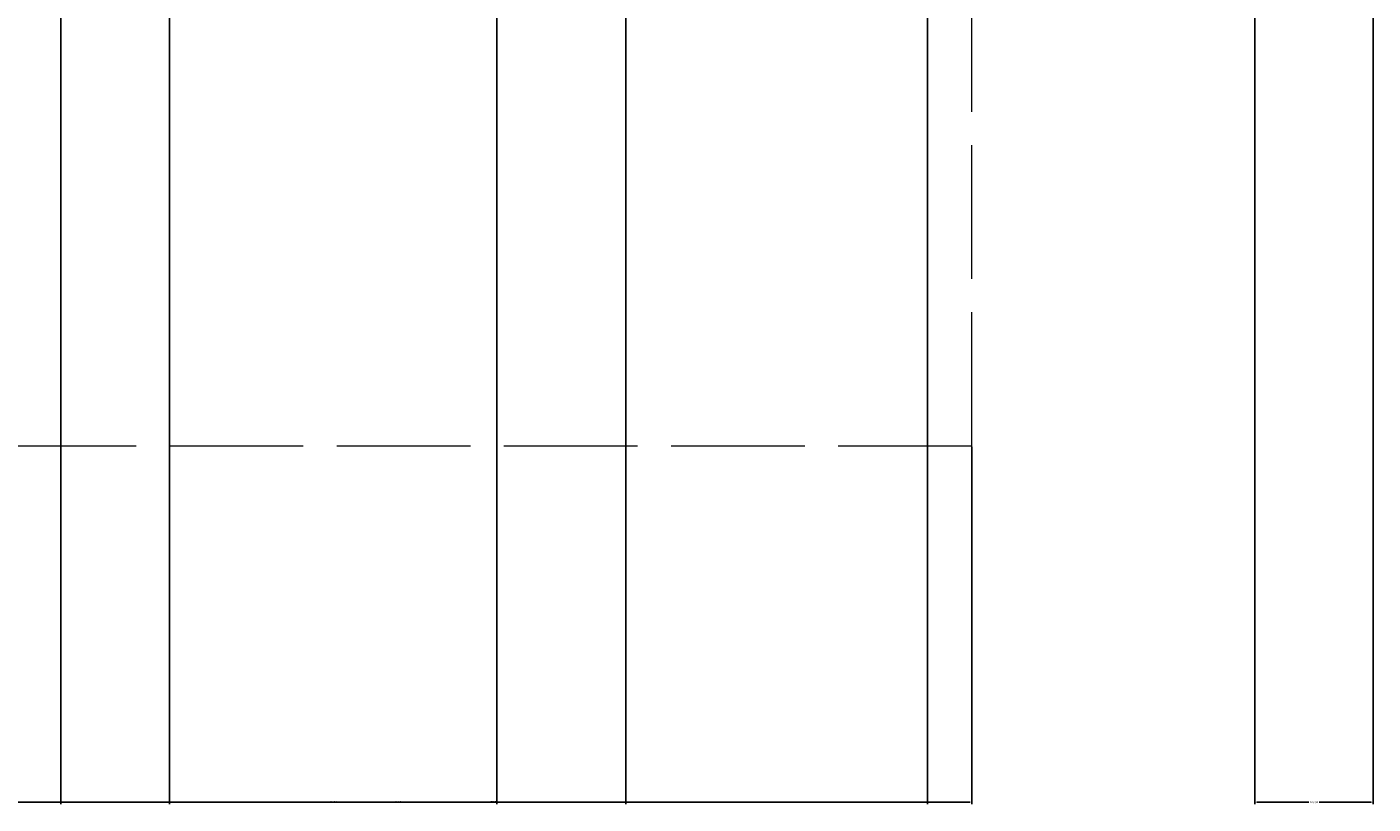
# Model space of a CAD drawing. Units: feet. Extents: x 1993 to 2298, y 2938 to 3641.
# Tile 2 of 11: x 2137 to 2258, y 2938 to 3008. Entities that reach past the tile are written whole.
import ezdxf

# ---------------------------------------------------------------- set-up
doc = ezdxf.new("R2010")
doc.units = ezdxf.units.FT
doc.linetypes.add('ACAD_ISO02W100', pattern=[15, 12, -3])
doc.layers.add('A-ANNO-DIMS', color=2, linetype='Continuous', lineweight=18)
doc.layers.add('SUNSHADES', color=4, linetype='ACAD_ISO02W100', lineweight=13)
doc.styles.get("Standard").update_dxf_attribs({"font": 'arial.ttf'})
doc.dimstyles.get("Standard").update_dxf_attribs({"dimtxt": 0.18, "dimasz": 0.18, "dimexe": 0.18, "dimexo": 0.0625, "dimgap": 0.09, "dimtad": 0, "dimtih": 1, "dimtoh": 1, "dimdec": 4, "dimzin": 0, "dimdsep": 46, "dimtxsty": 'Standard', "dimcen": 0.09, "dimadec": 0, "dimazin": 0, "dimtfac": 1, "dimtdec": 4, "dimtofl": 0, "dimtmove": 0, "dimatfit": 3, "dimfxl": 1, "dimtolj": 1, "dimtzin": 0, "dimarcsym": 0})

# ---------------------------------------------------------------- blocks, each defined once
blk = doc.blocks.new('*D57')
at = {"layer": 'A-ANNO-DIMS', "color": 0, "lineweight": -2, "transparency": 16777216}
for p, q in [((2029.76, 2969.94), (2029.76, 2937.86)), ((2221.76, 2969.94), (2221.76, 2937.86)), ((2029.94, 2938.03), (2125.48, 2938.03)), ((2221.58, 2938.03), (2126.04, 2938.03))]:
    blk.add_line(p, q, dxfattribs=at)
at = {"layer": 'A-ANNO-DIMS', "color": 0, "transparency": 16777216}
for points in [[(2029.94, 2938.07), (2029.94, 2938.01), (2029.76, 2938.03)], [(2221.58, 2938.07), (2221.58, 2938.01), (2221.76, 2938.03)]]:
    blk.add_solid(points, dxfattribs=at)
at = {"layer": 'Defpoints', "color": 0, "transparency": 16777216}
for p in [(2029.76, 2970), (2221.76, 2970), (2221.76, 2938.03)]:
    blk.add_point(p, dxfattribs=at)
at = {"layer": 'A-ANNO-DIMS', "color": 0, "transparency": 16777216, "insert": (2125.76, 2938.03), "char_height": 0.18, "attachment_point": 5}
blk.add_mtext('\\A1;192', dxfattribs=at)
blk = doc.blocks.new('*D60')
at = {"layer": 'A-ANNO-DIMS', "color": 0, "lineweight": -2, "transparency": 16777216}
for p, q in [((2140, 3012.47), (2140, 2937.86)), ((2217.76, 3012.47), (2217.76, 2937.86)), ((2140.18, 2938.03), (2178.49, 2938.03)), ((2217.58, 2938.03), (2179.27, 2938.03))]:
    blk.add_line(p, q, dxfattribs=at)
at = {"layer": 'A-ANNO-DIMS', "color": 0, "transparency": 16777216}
for points in [[(2140.18, 2938.07), (2140.18, 2938.01), (2140, 2938.03)], [(2217.58, 2938.07), (2217.58, 2938.01), (2217.76, 2938.03)]]:
    blk.add_solid(points, dxfattribs=at)
at = {"layer": 'Defpoints', "color": 0, "transparency": 16777216}
for p in [(2140, 3012.53), (2217.76, 3012.53), (2217.76, 2938.03)]:
    blk.add_point(p, dxfattribs=at)
at = {"layer": 'A-ANNO-DIMS', "color": 0, "transparency": 16777216, "insert": (2178.88, 2938.03), "char_height": 0.18, "attachment_point": 5}
blk.add_mtext('\\A1;77.76', dxfattribs=at)
blk = doc.blocks.new('*D65')
at = {"layer": 'A-ANNO-DIMS', "color": 0, "lineweight": -2, "transparency": 16777216}
for p, q in [((2179.12, 3231.85), (2179.12, 2937.86)), ((2149.76, 3228.47), (2149.76, 2937.86)), ((2149.94, 2938.03), (2164.04, 2938.03)), ((2178.94, 2938.03), (2164.83, 2938.03))]:
    blk.add_line(p, q, dxfattribs=at)
at = {"layer": 'A-ANNO-DIMS', "color": 0, "transparency": 16777216}
for points in [[(2149.94, 2938.07), (2149.94, 2938.01), (2149.76, 2938.03)], [(2178.94, 2938.07), (2178.94, 2938.01), (2179.12, 2938.03)]]:
    blk.add_solid(points, dxfattribs=at)
at = {"layer": 'Defpoints', "color": 0, "transparency": 16777216}
for p in [(2179.12, 3231.92), (2149.76, 3228.53), (2179.12, 2938.03)]:
    blk.add_point(p, dxfattribs=at)
at = {"layer": 'A-ANNO-DIMS', "color": 0, "transparency": 16777216, "insert": (2164.44, 2938.03), "char_height": 0.18, "attachment_point": 5}
blk.add_mtext('\\A1;29.36', dxfattribs=at)
blk = doc.blocks.new('*D66')
at = {"layer": 'A-ANNO-DIMS', "color": 0, "lineweight": -2, "transparency": 16777216}
for p, q in [((2247.15, 3235.34), (2247.15, 2937.86)), ((2257.76, 3228.47), (2257.76, 2937.86)), ((2247.33, 2938.03), (2252, 2938.03)), ((2257.58, 2938.03), (2252.91, 2938.03))]:
    blk.add_line(p, q, dxfattribs=at)
at = {"layer": 'A-ANNO-DIMS', "color": 0, "transparency": 16777216}
for points in [[(2247.33, 2938.07), (2247.33, 2938.01), (2247.15, 2938.03)], [(2257.58, 2938.07), (2257.58, 2938.01), (2257.76, 2938.03)]]:
    blk.add_solid(points, dxfattribs=at)
at = {"layer": 'Defpoints', "color": 0, "transparency": 16777216}
for p in [(2247.15, 3235.4), (2257.76, 3228.53), (2257.76, 2938.03)]:
    blk.add_point(p, dxfattribs=at)
at = {"layer": 'A-ANNO-DIMS', "color": 0, "transparency": 16777216, "insert": (2252.45, 2938.03), "char_height": 0.18, "attachment_point": 5}
blk.add_mtext('\\A1;10.608', dxfattribs=at)
blk = doc.blocks.new('*D69')
at = {"layer": 'A-ANNO-DIMS', "color": 0, "lineweight": -2, "transparency": 16777216}
for p, q in [((2149.76, 3492.27), (2149.76, 2937.86)), ((2190.69, 3492.27), (2190.69, 2937.86)), ((2149.94, 2938.03), (2169.83, 2938.03)), ((2190.51, 2938.03), (2170.62, 2938.03))]:
    blk.add_line(p, q, dxfattribs=at)
at = {"layer": 'A-ANNO-DIMS', "color": 0, "transparency": 16777216}
for points in [[(2149.94, 2938.07), (2149.94, 2938.01), (2149.76, 2938.03)], [(2190.51, 2938.07), (2190.51, 2938.01), (2190.69, 2938.03)]]:
    blk.add_solid(points, dxfattribs=at)
at = {"layer": 'Defpoints', "color": 0, "transparency": 16777216}
for p in [(2149.76, 3492.33), (2190.69, 3492.33), (2190.69, 2938.03)]:
    blk.add_point(p, dxfattribs=at)
at = {"layer": 'A-ANNO-DIMS', "color": 0, "transparency": 16777216, "insert": (2170.23, 2938.03), "char_height": 0.18, "attachment_point": 5}
blk.add_mtext('\\A1;40.93', dxfattribs=at)

msp = doc.modelspace()

# ---------------------------------------------------------------- linework, layer by layer
at = {"layer": 'SUNSHADES'}
for p, q in [((2221.7583, 2970), (2221.7583, 3010.5338)), ((2029.7583, 2970), (2221.7583, 2970))]:
    msp.add_line(p, q, dxfattribs=at)

# ---------------------------------------------------------------- dimensions: what is measured, and where the dimension line sits
at = {"layer": 'A-ANNO-DIMS'}
for base, p1, p2, override, picture, middle in [((2190.6917, 2938.035), (2149.7583, 3492.3338), (2190.6917, 3492.3338), {"dimdec": 2, "dimlfac": 1, "dimrnd": 0, "dimzin": 0, "dimdsep": 46, "dimlunit": 2}, '*D69', (2170.225, 2938.035)), ((2257.7583, 2938.035), (2247.1506, 3235.4), (2257.7583, 3228.5338), {"dimdec": 3, "dimlfac": 1, "dimrnd": 0, "dimzin": 0, "dimdsep": 46, "dimlunit": 2}, '*D66', (2252.4545, 2938.035)), ((2179.1188, 2938.035), (2149.7583, 3228.5338), (2179.1188, 3231.9167), {"dimdec": 2, "dimlfac": 1, "dimrnd": 0, "dimzin": 0, "dimdsep": 46, "dimlunit": 2}, '*D65', (2164.4386, 2938.035)), ((2217.7583, 2938.035), (2140, 3012.5338), (2217.7583, 3012.5338), {"dimdec": 2, "dimlfac": 1, "dimrnd": 0, "dimzin": 0, "dimdsep": 46, "dimlunit": 2}, '*D60', (2178.8792, 2938.035)), ((2221.7583, 2938.035), (2029.7583, 2970), (2221.7583, 2970), {"dimdec": 0, "dimlfac": 1, "dimrnd": 0, "dimzin": 0, "dimdsep": 46, "dimlunit": 2}, '*D57', (2125.7583, 2938.035))]:
    dim = msp.add_linear_dim(base=base, p1=p1, p2=p2, dimstyle='Standard', override=override, dxfattribs=at)
    dim.commit()
    dim.dimension.update_dxf_attribs({"geometry": picture, "text_midpoint": middle})

doc.saveas('drawing.dxf')
